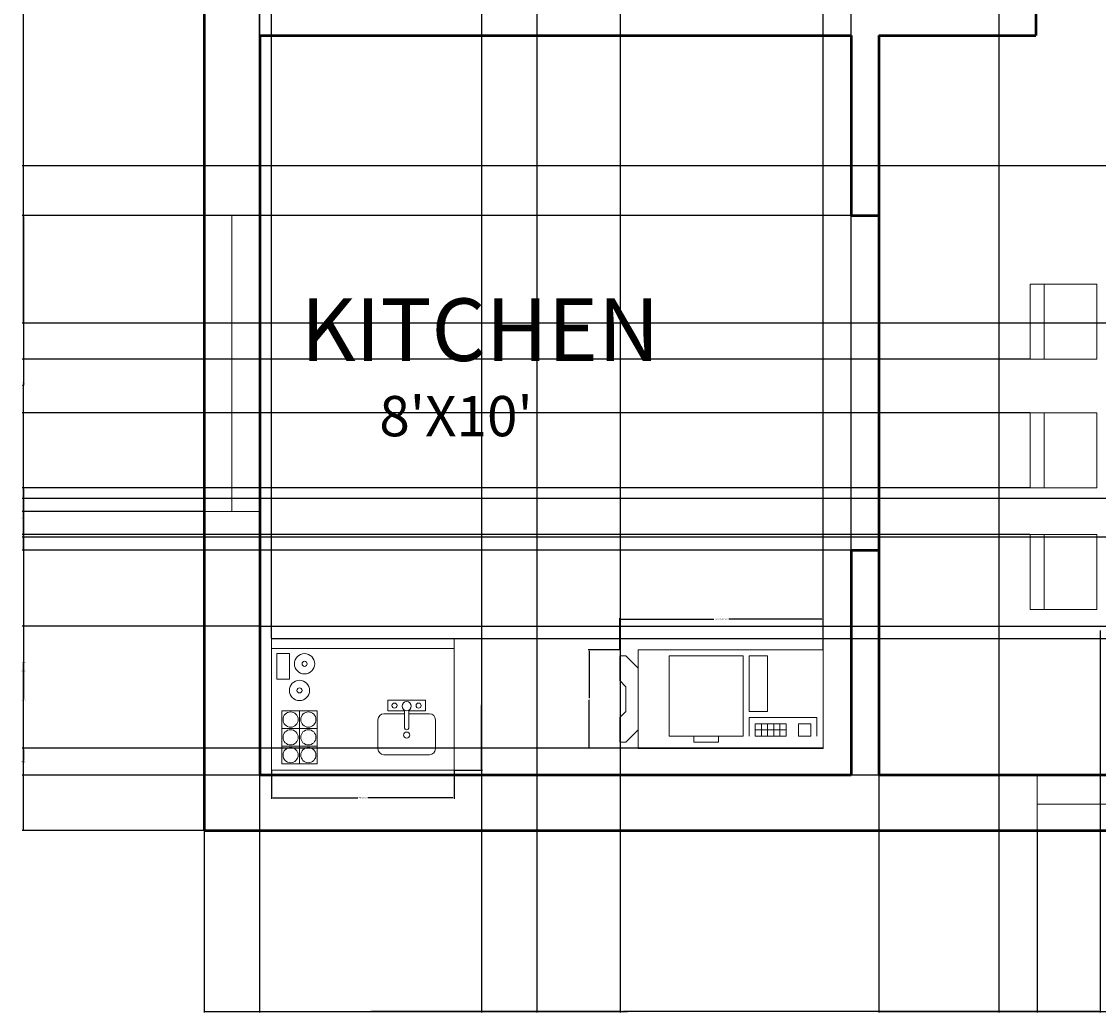
# Model space of a CAD drawing. Units: inches. Extents: x 19425 to 19848, y 45806 to 46417.
# Tile 1 of 5: x 19425 to 19600, y 45806 to 45967. Entities that reach past the tile are written whole.
import ezdxf

# ---------------------------------------------------------------- set-up
doc = ezdxf.new("R2010")
doc.units = ezdxf.units.IN
for name, color, linetype, lineweight in [('A-ANNO-DIMS', 2, 'Continuous', 18), ('A-AREA-IDEN', 3, 'Continuous', 25), ('A-EQPM', 2, 'Continuous', 18), ('A-FLOR-CASE', 2, 'Continuous', 20), ('A-FLOR-FIXT', 2, 'Continuous', 20), ('furniture', 2, 'Continuous', 18), ('wall', 6, 'Continuous', 50), ('window', 9, 'Continuous', 20)]:
    doc.layers.add(name, color=color, linetype=linetype, lineweight=lineweight)
doc.styles.get("Standard").update_dxf_attribs({"font": 'arial.ttf'})
doc.dimstyles.get("Standard").update_dxf_attribs({"dimtxt": 0.18, "dimasz": 0.18, "dimexe": 0.18, "dimexo": 0.0625, "dimgap": 0.09, "dimtad": 0, "dimtih": 1, "dimtoh": 1, "dimdec": 4, "dimzin": 0, "dimdsep": 46, "dimtxsty": 'Standard', "dimcen": 0.09, "dimadec": 0, "dimazin": 0, "dimtfac": 1, "dimtdec": 4, "dimtofl": 0, "dimtmove": 0, "dimatfit": 3, "dimfxl": 1, "dimtolj": 1, "dimtzin": 0, "dimarcsym": 0})

# ---------------------------------------------------------------- blocks, each defined once
blk = doc.blocks.new('Copy Machine')
for p, q in [((0, 0), (0, -16)), ((30, 0), (0, 0)), ((30, -16), (30, 0)), ((-3, -1), (-3, -5)), ((-2, -1), (-3, -1)), ((0, -3), (-2, -1)), ((5, -1), (5, -14)), ((17, -1), (5, -1)), ((17, -14), (17, -1)), ((18, -1), (18, -10)), ((21, -1), (18, -1)), ((21, -10), (21, -1)), ((-3, -5), (-2, -6)), ((-2, -10), (-2, -6)), ((-3, -11), (-2, -10)), ((18, -10), (21, -10)), ((-3, -15), (-3, -11)), ((18, -14), (18, -11)), ((18, -11), (29, -11)), ((24, -12), (19, -12)), ((19, -12), (19, -14)), ((20, -12), (20, -14)), ((21, -14), (21, -12)), ((22, -12), (22, -14)), ((23, -14), (23, -12)), ((24, -14), (24, -12)), ((28, -12), (26, -12)), ((26, -12), (26, -14)), ((28, -14), (28, -12)), ((29, -11), (29, -14)), ((0, -13), (-2, -15)), ((24, -13), (19, -13)), ((-2, -15), (-3, -15)), ((5, -14), (17, -14)), ((9, -14), (9, -15)), ((9, -15), (13, -15)), ((13, -15), (13, -14)), ((19, -14), (24, -14)), ((26, -14), (28, -14)), ((0, -16), (30, -16))]:
    blk.add_line(p, q)
blk = doc.blocks.new('Wet Bar')
for p, q in [((0, 0), (36, 0)), ((0, -26), (0, 0)), ((36, 0), (36, -26)), ((0, -2), (36, -2)), ((3.5, -3), (1, -3)), ((1, -3), (1, -8)), ((3.5, -8), (3.5, -3)), ((1, -8), (3.5, -8)), ((2, -14.25), (9, -14.25)), ((2, -24.75), (2, -14.25)), ((5.5, -14.25), (5.5, -24.75)), ((9, -14.25), (9, -24.75)), ((26.2, -17.55), (26.2, -14.1284)), ((27.1001, -17.55), (27.1001, -14.1284)), ((2, -17.75), (9, -17.75)), ((9, -21.25), (2, -21.25)), ((9, -24.75), (2, -24.75)), ((36, -26), (0, -26))]:
    blk.add_line(p, q)
for points in [[(26.2, -14.25), (22.95, -14.25), (22.95, -12.2), (26.75, -12.2)], [(26.7487, -12.2), (30.3501, -12.2), (30.3501, -14.25), (27.1001, -14.25)], [(22.15, -14.85), (26.2, -14.85)], [(27.1001, -14.85), (31.15, -14.85)], [(20.95, -21.75), (20.95, -16.05)], [(32.3501, -16.05), (32.3501, -21.75)], [(31.15, -22.95), (22.15, -22.95)]]:
    blk.add_lwpolyline(points)
for centre, radius in [((6.5, -5), 2), ((6.5, -5), 0.5), ((5.5, -10.25), 2), ((5.5, -10.25), 0.5), ((26.65, -13.35), 0.9), ((3.75, -16), 1.5), ((7.25, -16), 1.5), ((24.25, -13.25), 0.5), ((29, -13.25), 0.5), ((3.75, -19.5), 1.5), ((7.25, -19.5), 1.5), ((26.65, -19.05), 0.6), ((3.75, -23), 1.5), ((7.25, -23), 1.5)]:
    blk.add_circle(centre, radius)
for centre, radius, start, end in [((22.2251, -16.125), 1.2772, 93.36646, 176.6335), ((31.075, -16.125), 1.2772, 3.366461, 86.63354), ((26.65, -17.55), 0.45, 180, 0), ((22.2251, -21.675), 1.2772, 183.3665, 266.6335), ((31.075, -21.675), 1.2772, 273.3665, 356.6335)]:
    blk.add_arc(centre, radius, start, end)
blk = doc.blocks.new('WIN-48-CENTER-9')
for p, q in [((0, 48), (9, 48)), ((4.5, 0), (4.5, 48)), ((0, 0), (9, 0))]:
    blk.add_line(p, q)
blk = doc.blocks.new('WIN-48-OFFSET-9')
for p, q in [((0, 0), (0, 9)), ((48, 0), (48, 9)), ((48, 4.28), (0, 4.28))]:
    blk.add_line(p, q)
blk = doc.blocks.new('CHAIR-DINING')
blk.add_line((0, 8.53), (12.17, 8.53))
blk.add_lwpolyline([(0, 10.82), (12.17, 10.82), (12.17, 0), (0, 0)], close=True)
blk = doc.blocks.new('*D28')
at = {"layer": 'A-ANNO-DIMS', "color": 0, "lineweight": -2, "transparency": 16777216}
for p, q in [((19522.24, 45865.14), (19522.24, 45870.21)), ((19522.42, 45870.03), (19537.52, 45870.03)), ((19555.06, 45870.03), (19539.96, 45870.03)), ((19555.24, 45865.14), (19555.24, 45870.21))]:
    blk.add_line(p, q, dxfattribs=at)
at = {"layer": 'A-ANNO-DIMS', "color": 0, "transparency": 16777216}
for points in [[(19522.42, 45870.06), (19522.42, 45870), (19522.24, 45870.03)], [(19555.06, 45870.06), (19555.06, 45870), (19555.24, 45870.03)]]:
    blk.add_solid(points, dxfattribs=at)
at = {"layer": 'Defpoints', "color": 0, "transparency": 16777216}
for p in [(19555.24, 45870.03), (19522.24, 45865.08), (19555.24, 45865.08)]:
    blk.add_point(p, dxfattribs=at)
at = {"layer": 'A-ANNO-DIMS', "color": 0, "transparency": 16777216, "insert": (19538.74, 45870.03), "char_height": 0.18, "attachment_point": 5}
blk.add_mtext('\\A1;COPY MACHINE 33', dxfattribs=at)
blk = doc.blocks.new('*D29')
at = {"layer": 'A-ANNO-DIMS', "color": 0, "lineweight": -2, "transparency": 16777216}
for p, q in [((19522.18, 45865.08), (19517.11, 45865.08)), ((19517.29, 45864.9), (19517.29, 45857.26)), ((19517.29, 45849.26), (19517.29, 45856.89)), ((19522.18, 45849.08), (19517.11, 45849.08))]:
    blk.add_line(p, q, dxfattribs=at)
at = {"layer": 'A-ANNO-DIMS', "color": 0, "transparency": 16777216}
for points in [[(19517.26, 45864.9), (19517.32, 45864.9), (19517.29, 45865.08)], [(19517.26, 45849.26), (19517.32, 45849.26), (19517.29, 45849.08)]]:
    blk.add_solid(points, dxfattribs=at)
at = {"layer": 'Defpoints', "color": 0, "transparency": 16777216}
for p in [(19517.29, 45865.08), (19522.24, 45865.08), (19522.24, 45849.08)]:
    blk.add_point(p, dxfattribs=at)
at = {"layer": 'A-ANNO-DIMS', "color": 0, "transparency": 16777216, "insert": (19517.29, 45857.08), "char_height": 0.18, "attachment_point": 5}
blk.add_mtext('\\A1;16', dxfattribs=at)
blk = doc.blocks.new('*D30')
at = {"layer": 'A-ANNO-DIMS', "color": 0, "lineweight": -2, "transparency": 16777216}
for p, q in [((19465.72, 45845.46), (19465.72, 45840.89)), ((19495.34, 45845.46), (19495.34, 45840.89)), ((19465.9, 45841.07), (19479.7, 45841.07)), ((19495.16, 45841.07), (19481.36, 45841.07))]:
    blk.add_line(p, q, dxfattribs=at)
at = {"layer": 'A-ANNO-DIMS', "color": 0, "transparency": 16777216}
for points in [[(19465.9, 45841.1), (19465.9, 45841.04), (19465.72, 45841.07)], [(19495.16, 45841.1), (19495.16, 45841.04), (19495.34, 45841.07)]]:
    blk.add_solid(points, dxfattribs=at)
at = {"layer": 'Defpoints', "color": 0, "transparency": 16777216}
for p in [(19465.72, 45845.52), (19495.34, 45845.52), (19495.34, 45841.07)]:
    blk.add_point(p, dxfattribs=at)
at = {"layer": 'A-ANNO-DIMS', "color": 0, "transparency": 16777216, "insert": (19480.53, 45841.07), "char_height": 0.18, "attachment_point": 5}
blk.add_mtext('\\A1;WET BAR 30', dxfattribs=at)
blk = doc.blocks.new('*D31')
at = {"layer": 'A-ANNO-DIMS', "color": 0, "lineweight": -2, "transparency": 16777216}
for p, q in [((19495.4, 45866.91), (19499.96, 45866.91)), ((19499.78, 45866.73), (19499.78, 45856.39)), ((19499.78, 45845.7), (19499.78, 45856.03)), ((19495.4, 45845.52), (19499.96, 45845.52))]:
    blk.add_line(p, q, dxfattribs=at)
at = {"layer": 'A-ANNO-DIMS', "color": 0, "transparency": 16777216}
for points in [[(19499.75, 45866.73), (19499.81, 45866.73), (19499.78, 45866.91)], [(19499.75, 45845.7), (19499.81, 45845.7), (19499.78, 45845.52)]]:
    blk.add_solid(points, dxfattribs=at)
at = {"layer": 'Defpoints', "color": 0, "transparency": 16777216}
for p in [(19495.34, 45866.91), (19499.78, 45866.91), (19495.34, 45845.52)]:
    blk.add_point(p, dxfattribs=at)
at = {"layer": 'A-ANNO-DIMS', "color": 0, "transparency": 16777216, "insert": (19499.78, 45856.21), "char_height": 0.18, "attachment_point": 5}
blk.add_mtext('\\A1;21', dxfattribs=at)
blk = doc.blocks.new('*D34')
at = {"layer": 'A-ANNO-DIMS', "color": 0, "lineweight": -2, "transparency": 16777216}
for p, q in [((19522.3, 46304.14), (19522.3, 45806.22)), ((19463.78, 46303.69), (19463.78, 45806.22)), ((19463.96, 45806.4), (19492.65, 45806.4)), ((19522.12, 45806.4), (19493.43, 45806.4))]:
    blk.add_line(p, q, dxfattribs=at)
at = {"layer": 'A-ANNO-DIMS', "color": 0, "transparency": 16777216}
for points in [[(19463.96, 45806.43), (19463.96, 45806.37), (19463.78, 45806.4)], [(19522.12, 45806.43), (19522.12, 45806.37), (19522.3, 45806.4)]]:
    blk.add_solid(points, dxfattribs=at)
at = {"layer": 'Defpoints', "color": 0, "transparency": 16777216}
for p in [(19522.3, 46304.2), (19463.78, 46303.75), (19522.3, 45806.4)]:
    blk.add_point(p, dxfattribs=at)
at = {"layer": 'A-ANNO-DIMS', "color": 0, "transparency": 16777216, "insert": (19493.04, 45806.4), "char_height": 0.18, "attachment_point": 5}
blk.add_mtext('\\A1;58.52', dxfattribs=at)
blk = doc.blocks.new('*D37')
at = {"layer": 'A-ANNO-DIMS', "color": 0, "lineweight": -2, "transparency": 16777216}
for p, q in [((19454.72, 45887.51), (19425.25, 45887.51)), ((19425.43, 45887.33), (19425.43, 45861.82)), ((19425.43, 45835.93), (19425.43, 45861.45)), ((19454.72, 45835.75), (19425.25, 45835.75))]:
    blk.add_line(p, q, dxfattribs=at)
at = {"layer": 'A-ANNO-DIMS', "color": 0, "transparency": 16777216}
for points in [[(19425.4, 45887.33), (19425.46, 45887.33), (19425.43, 45887.51)], [(19425.4, 45835.93), (19425.46, 45835.93), (19425.43, 45835.75)]]:
    blk.add_solid(points, dxfattribs=at)
at = {"layer": 'Defpoints', "color": 0, "transparency": 16777216}
for p in [(19425.43, 45887.51), (19454.78, 45887.51), (19454.78, 45835.75)]:
    blk.add_point(p, dxfattribs=at)
at = {"layer": 'A-ANNO-DIMS', "color": 0, "transparency": 16777216, "insert": (19425.43, 45861.63), "char_height": 0.18, "attachment_point": 5}
blk.add_mtext('\\A1;51.76', dxfattribs=at)
blk = doc.blocks.new('*D38')
at = {"layer": 'A-ANNO-DIMS', "color": 0, "lineweight": -2, "transparency": 16777216}
for p, q in [((19808.72, 45889.62), (19425.25, 45889.62)), ((19425.43, 45889.44), (19425.43, 45886.67)), ((19425.43, 45883.53), (19425.43, 45886.3)), ((19802.72, 45883.35), (19425.25, 45883.35))]:
    blk.add_line(p, q, dxfattribs=at)
at = {"layer": 'A-ANNO-DIMS', "color": 0, "transparency": 16777216}
for points in [[(19425.4, 45889.44), (19425.46, 45889.44), (19425.43, 45889.62)], [(19425.4, 45883.53), (19425.46, 45883.53), (19425.43, 45883.35)]]:
    blk.add_solid(points, dxfattribs=at)
at = {"layer": 'Defpoints', "color": 0, "transparency": 16777216}
for p in [(19425.43, 45889.62), (19808.78, 45889.62), (19802.78, 45883.35)]:
    blk.add_point(p, dxfattribs=at)
at = {"layer": 'A-ANNO-DIMS', "color": 0, "transparency": 16777216, "insert": (19425.43, 45886.49), "char_height": 0.18, "attachment_point": 5}
blk.add_mtext('\\A1;6.261', dxfattribs=at)
blk = doc.blocks.new('*D39')
at = {"layer": 'A-ANNO-DIMS', "color": 0, "lineweight": -2, "transparency": 16777216}
for p, q in [((19454.78, 45835.69), (19454.78, 45806.22)), ((19590, 45835.69), (19590, 45806.22)), ((19454.96, 45806.4), (19521.93, 45806.4)), ((19589.82, 45806.4), (19522.84, 45806.4))]:
    blk.add_line(p, q, dxfattribs=at)
at = {"layer": 'A-ANNO-DIMS', "color": 0, "transparency": 16777216}
for points in [[(19454.96, 45806.43), (19454.96, 45806.37), (19454.78, 45806.4)], [(19589.82, 45806.43), (19589.82, 45806.37), (19590, 45806.4)]]:
    blk.add_solid(points, dxfattribs=at)
at = {"layer": 'Defpoints', "color": 0, "transparency": 16777216}
for p in [(19454.78, 45835.75), (19590, 45835.75), (19590, 45806.4)]:
    blk.add_point(p, dxfattribs=at)
at = {"layer": 'A-ANNO-DIMS', "color": 0, "transparency": 16777216, "insert": (19522.39, 45806.4), "char_height": 0.18, "attachment_point": 5}
blk.add_mtext('\\A1;135.22', dxfattribs=at)
blk = doc.blocks.new('*D43')
at = {"layer": 'A-ANNO-DIMS', "color": 0, "lineweight": -2, "transparency": 16777216}
for p, q in [((19564.28, 45844.69), (19564.28, 45806.22)), ((19666.28, 45844.69), (19666.28, 45806.22)), ((19564.46, 45806.4), (19615, 45806.4)), ((19666.1, 45806.4), (19615.56, 45806.4))]:
    blk.add_line(p, q, dxfattribs=at)
at = {"layer": 'A-ANNO-DIMS', "color": 0, "transparency": 16777216}
for points in [[(19564.46, 45806.43), (19564.46, 45806.37), (19564.28, 45806.4)], [(19666.1, 45806.43), (19666.1, 45806.37), (19666.28, 45806.4)]]:
    blk.add_solid(points, dxfattribs=at)
at = {"layer": 'Defpoints', "color": 0, "transparency": 16777216}
for p in [(19564.28, 45844.75), (19666.28, 45844.75), (19666.28, 45806.4)]:
    blk.add_point(p, dxfattribs=at)
at = {"layer": 'A-ANNO-DIMS', "color": 0, "transparency": 16777216, "insert": (19615.28, 45806.4), "char_height": 0.18, "attachment_point": 5}
blk.add_mtext('\\A1;102', dxfattribs=at)
blk = doc.blocks.new('*D48')
at = {"layer": 'A-ANNO-DIMS', "color": 0, "lineweight": -2, "transparency": 16777216}
for p, q in [((19564.22, 45935.54), (19425.25, 45935.54)), ((19425.43, 45935.36), (19425.43, 45908.56)), ((19425.43, 45881.4), (19425.43, 45908.19)), ((19564.22, 45881.22), (19425.25, 45881.22))]:
    blk.add_line(p, q, dxfattribs=at)
at = {"layer": 'A-ANNO-DIMS', "color": 0, "transparency": 16777216}
for points in [[(19425.4, 45935.36), (19425.46, 45935.36), (19425.43, 45935.54)], [(19425.4, 45881.4), (19425.46, 45881.4), (19425.43, 45881.22)]]:
    blk.add_solid(points, dxfattribs=at)
at = {"layer": 'Defpoints', "color": 0, "transparency": 16777216}
for p in [(19425.43, 45935.54), (19564.28, 45935.54), (19564.28, 45881.22)]:
    blk.add_point(p, dxfattribs=at)
at = {"layer": 'A-ANNO-DIMS', "color": 0, "transparency": 16777216, "insert": (19425.43, 45908.38), "char_height": 0.18, "attachment_point": 5}
blk.add_mtext('\\A1;54.32', dxfattribs=at)
blk = doc.blocks.new('*D52')
at = {"layer": 'A-ANNO-DIMS', "color": 0, "lineweight": -2, "transparency": 16777216}
for p, q in [((19732.81, 46000.63), (19425.25, 46000.63)), ((19425.43, 46000.45), (19425.43, 45972.3)), ((19425.43, 45943.79), (19425.43, 45971.94)), ((19732.81, 45943.61), (19425.25, 45943.61))]:
    blk.add_line(p, q, dxfattribs=at)
at = {"layer": 'A-ANNO-DIMS', "color": 0, "transparency": 16777216}
for points in [[(19425.4, 46000.45), (19425.46, 46000.45), (19425.43, 46000.63)], [(19425.4, 45943.79), (19425.46, 45943.79), (19425.43, 45943.61)]]:
    blk.add_solid(points, dxfattribs=at)
at = {"layer": 'Defpoints', "color": 0, "transparency": 16777216}
for p in [(19425.43, 46000.63), (19732.87, 46000.63), (19732.87, 45943.61)]:
    blk.add_point(p, dxfattribs=at)
at = {"layer": 'A-ANNO-DIMS', "color": 0, "transparency": 16777216, "insert": (19425.43, 45972.12), "char_height": 0.18, "attachment_point": 5}
blk.add_mtext('\\A1;57.02', dxfattribs=at)
blk = doc.blocks.new('*D54')
at = {"layer": 'A-ANNO-DIMS', "color": 0, "lineweight": -2, "transparency": 16777216}
for p, q in [((19808.72, 46048.75), (19425.25, 46048.75)), ((19425.43, 46048.57), (19425.43, 45983.58)), ((19425.43, 45918.22), (19425.43, 45983.22)), ((19808.72, 45918.04), (19425.25, 45918.04))]:
    blk.add_line(p, q, dxfattribs=at)
at = {"layer": 'A-ANNO-DIMS', "color": 0, "transparency": 16777216}
for points in [[(19425.4, 46048.57), (19425.46, 46048.57), (19425.43, 46048.75)], [(19425.4, 45918.22), (19425.46, 45918.22), (19425.43, 45918.04)]]:
    blk.add_solid(points, dxfattribs=at)
at = {"layer": 'Defpoints', "color": 0, "transparency": 16777216}
for p in [(19425.43, 46048.75), (19808.78, 46048.75), (19808.78, 45918.04)]:
    blk.add_point(p, dxfattribs=at)
at = {"layer": 'A-ANNO-DIMS', "color": 0, "transparency": 16777216, "insert": (19425.43, 45983.4), "char_height": 0.18, "attachment_point": 5}
blk.add_mtext('\\A1;130.7', dxfattribs=at)
blk = doc.blocks.new('*D56')
at = {"layer": 'A-ANNO-DIMS', "color": 0, "lineweight": -2, "transparency": 16777216}
for p, q in [((19564.28, 45881.15), (19564.28, 45806.22)), ((19600.2, 45868.22), (19600.2, 45806.22)), ((19564.46, 45806.4), (19581.85, 45806.4)), ((19600.02, 45806.4), (19582.63, 45806.4))]:
    blk.add_line(p, q, dxfattribs=at)
at = {"layer": 'A-ANNO-DIMS', "color": 0, "transparency": 16777216}
for points in [[(19564.46, 45806.43), (19564.46, 45806.37), (19564.28, 45806.4)], [(19600.02, 45806.43), (19600.02, 45806.37), (19600.2, 45806.4)]]:
    blk.add_solid(points, dxfattribs=at)
at = {"layer": 'Defpoints', "color": 0, "transparency": 16777216}
for p in [(19564.28, 45881.22), (19600.2, 45868.28), (19600.2, 45806.4)]:
    blk.add_point(p, dxfattribs=at)
at = {"layer": 'A-ANNO-DIMS', "color": 0, "transparency": 16777216, "insert": (19582.24, 45806.4), "char_height": 0.18, "attachment_point": 5}
blk.add_mtext('\\A1;35.92', dxfattribs=at)
blk = doc.blocks.new('*D58')
at = {"layer": 'A-ANNO-DIMS', "color": 0, "lineweight": -2, "transparency": 16777216}
for p, q in [((19463.72, 45868.92), (19425.25, 45868.92)), ((19425.43, 45868.74), (19425.43, 45857.02)), ((19425.43, 45844.93), (19425.43, 45856.65)), ((19463.72, 45844.75), (19425.25, 45844.75))]:
    blk.add_line(p, q, dxfattribs=at)
at = {"layer": 'A-ANNO-DIMS', "color": 0, "transparency": 16777216}
for points in [[(19425.4, 45868.74), (19425.46, 45868.74), (19425.43, 45868.92)], [(19425.4, 45844.93), (19425.46, 45844.93), (19425.43, 45844.75)]]:
    blk.add_solid(points, dxfattribs=at)
at = {"layer": 'Defpoints', "color": 0, "transparency": 16777216}
for p in [(19425.43, 45868.92), (19463.78, 45868.92), (19463.78, 45844.75)]:
    blk.add_point(p, dxfattribs=at)
at = {"layer": 'A-ANNO-DIMS', "color": 0, "transparency": 16777216, "insert": (19425.43, 45856.84), "char_height": 0.18, "attachment_point": 5}
blk.add_mtext('\\A1;24.16', dxfattribs=at)
blk = doc.blocks.new('*D59')
at = {"layer": 'A-ANNO-DIMS', "color": 0, "lineweight": -2, "transparency": 16777216}
for p, q in [((19463.78, 45868.98), (19463.78, 46342.28)), ((19463.96, 46342.1), (19464.36, 46342.1)), ((19465.54, 46342.1), (19465.14, 46342.1)), ((19465.72, 45866.97), (19465.72, 46342.28))]:
    blk.add_line(p, q, dxfattribs=at)
at = {"layer": 'A-ANNO-DIMS', "color": 0, "transparency": 16777216}
for points in [[(19463.96, 46342.13), (19463.96, 46342.07), (19463.78, 46342.1)], [(19465.54, 46342.13), (19465.54, 46342.07), (19465.72, 46342.1)]]:
    blk.add_solid(points, dxfattribs=at)
at = {"layer": 'Defpoints', "color": 0, "transparency": 16777216}
for p in [(19465.72, 46342.1), (19463.78, 45868.92), (19465.72, 45866.91)]:
    blk.add_point(p, dxfattribs=at)
at = {"layer": 'A-ANNO-DIMS', "color": 0, "transparency": 16777216, "insert": (19464.75, 46342.1), "char_height": 0.18, "attachment_point": 5}
blk.add_mtext('\\A1;1.938', dxfattribs=at)
blk = doc.blocks.new('*D60')
at = {"layer": 'A-ANNO-DIMS', "color": 0, "lineweight": -2, "transparency": 16777216}
for p, q in [((19555.24, 45865.14), (19555.24, 46342.28)), ((19555.42, 46342.1), (19557.18, 46342.1)), ((19559.6, 46342.1), (19557.84, 46342.1)), ((19559.78, 45868.98), (19559.78, 46342.28))]:
    blk.add_line(p, q, dxfattribs=at)
at = {"layer": 'A-ANNO-DIMS', "color": 0, "transparency": 16777216}
for points in [[(19555.42, 46342.13), (19555.42, 46342.07), (19555.24, 46342.1)], [(19559.6, 46342.13), (19559.6, 46342.07), (19559.78, 46342.1)]]:
    blk.add_solid(points, dxfattribs=at)
at = {"layer": 'Defpoints', "color": 0, "transparency": 16777216}
for p in [(19559.78, 46342.1), (19559.78, 45868.92), (19555.24, 45865.08)]:
    blk.add_point(p, dxfattribs=at)
at = {"layer": 'A-ANNO-DIMS', "color": 0, "transparency": 16777216, "insert": (19557.51, 46342.1), "char_height": 0.18, "attachment_point": 5}
blk.add_mtext('\\A1;4.54', dxfattribs=at)
blk = doc.blocks.new('*D63')
at = {"layer": 'A-ANNO-DIMS', "color": 0, "lineweight": -2, "transparency": 16777216}
for p, q in [((19463.78, 46125.19), (19463.78, 45806.22)), ((19583.78, 46125.19), (19583.78, 45806.22)), ((19463.96, 45806.4), (19523.5, 45806.4)), ((19583.6, 45806.4), (19524.06, 45806.4))]:
    blk.add_line(p, q, dxfattribs=at)
at = {"layer": 'A-ANNO-DIMS', "color": 0, "transparency": 16777216}
for points in [[(19463.96, 45806.43), (19463.96, 45806.37), (19463.78, 45806.4)], [(19583.6, 45806.43), (19583.6, 45806.37), (19583.78, 45806.4)]]:
    blk.add_solid(points, dxfattribs=at)
at = {"layer": 'Defpoints', "color": 0, "transparency": 16777216}
for p in [(19463.78, 46125.25), (19583.78, 46125.25), (19583.78, 45806.4)]:
    blk.add_point(p, dxfattribs=at)
at = {"layer": 'A-ANNO-DIMS', "color": 0, "transparency": 16777216, "insert": (19523.78, 45806.4), "char_height": 0.18, "attachment_point": 5}
blk.add_mtext('\\A1;120', dxfattribs=at)
blk = doc.blocks.new('*D64')
at = {"layer": 'A-ANNO-DIMS', "color": 0, "lineweight": -2, "transparency": 16777216}
for p, q in [((19463.78, 46048.69), (19463.78, 45806.22)), ((19499.78, 46048.69), (19499.78, 45806.22)), ((19463.96, 45806.4), (19481.56, 45806.4)), ((19499.6, 45806.4), (19482, 45806.4))]:
    blk.add_line(p, q, dxfattribs=at)
at = {"layer": 'A-ANNO-DIMS', "color": 0, "transparency": 16777216}
for points in [[(19463.96, 45806.43), (19463.96, 45806.37), (19463.78, 45806.4)], [(19499.6, 45806.43), (19499.6, 45806.37), (19499.78, 45806.4)]]:
    blk.add_solid(points, dxfattribs=at)
at = {"layer": 'Defpoints', "color": 0, "transparency": 16777216}
for p in [(19463.78, 46048.75), (19499.78, 46048.75), (19499.78, 45806.4)]:
    blk.add_point(p, dxfattribs=at)
at = {"layer": 'A-ANNO-DIMS', "color": 0, "transparency": 16777216, "insert": (19481.78, 45806.4), "char_height": 0.18, "attachment_point": 5}
blk.add_mtext('\\A1;36', dxfattribs=at)
blk = doc.blocks.new('*D65')
at = {"layer": 'A-ANNO-DIMS', "color": 0, "lineweight": -2, "transparency": 16777216}
for p, q in [((19499.78, 46048.69), (19499.78, 45806.22)), ((19508.78, 46048.69), (19508.78, 45806.22)), ((19499.96, 45806.4), (19504.13, 45806.4)), ((19508.6, 45806.4), (19504.43, 45806.4))]:
    blk.add_line(p, q, dxfattribs=at)
at = {"layer": 'A-ANNO-DIMS', "color": 0, "transparency": 16777216}
for points in [[(19499.96, 45806.43), (19499.96, 45806.37), (19499.78, 45806.4)], [(19508.6, 45806.43), (19508.6, 45806.37), (19508.78, 45806.4)]]:
    blk.add_solid(points, dxfattribs=at)
at = {"layer": 'Defpoints', "color": 0, "transparency": 16777216}
for p in [(19499.78, 46048.75), (19508.78, 46048.75), (19508.78, 45806.4)]:
    blk.add_point(p, dxfattribs=at)
at = {"layer": 'A-ANNO-DIMS', "color": 0, "transparency": 16777216, "insert": (19504.28, 45806.4), "char_height": 0.18, "attachment_point": 5}
blk.add_mtext('\\A1;9', dxfattribs=at)
blk = doc.blocks.new('*D71')
at = {"layer": 'A-ANNO-DIMS', "color": 0, "lineweight": -2, "transparency": 16777216}
for p, q in [((19564.22, 45881.22), (19425.25, 45881.22)), ((19425.43, 45881.04), (19425.43, 45863.17)), ((19425.43, 45844.93), (19425.43, 45862.8)), ((19564.22, 45844.75), (19425.25, 45844.75))]:
    blk.add_line(p, q, dxfattribs=at)
at = {"layer": 'A-ANNO-DIMS', "color": 0, "transparency": 16777216}
for points in [[(19425.4, 45881.04), (19425.46, 45881.04), (19425.43, 45881.22)], [(19425.4, 45844.93), (19425.46, 45844.93), (19425.43, 45844.75)]]:
    blk.add_solid(points, dxfattribs=at)
at = {"layer": 'Defpoints', "color": 0, "transparency": 16777216}
for p in [(19425.43, 45881.22), (19564.28, 45881.22), (19564.28, 45844.75)]:
    blk.add_point(p, dxfattribs=at)
at = {"layer": 'A-ANNO-DIMS', "color": 0, "transparency": 16777216, "insert": (19425.43, 45862.99), "char_height": 0.18, "attachment_point": 5}
blk.add_mtext('\\A1;36.46', dxfattribs=at)
blk = doc.blocks.new('*D72')
at = {"layer": 'A-ANNO-DIMS', "color": 0, "lineweight": -2, "transparency": 16777216}
for p, q in [((19588.8, 45912.22), (19425.25, 45912.22)), ((19425.43, 45912.04), (19425.43, 45908.06)), ((19425.43, 45903.71), (19425.43, 45907.7)), ((19588.8, 45903.53), (19425.25, 45903.53))]:
    blk.add_line(p, q, dxfattribs=at)
at = {"layer": 'A-ANNO-DIMS', "color": 0, "transparency": 16777216}
for points in [[(19425.4, 45912.04), (19425.46, 45912.04), (19425.43, 45912.22)], [(19425.4, 45903.71), (19425.46, 45903.71), (19425.43, 45903.53)]]:
    blk.add_solid(points, dxfattribs=at)
at = {"layer": 'Defpoints', "color": 0, "transparency": 16777216}
for p in [(19425.43, 45912.22), (19588.86, 45912.22), (19588.86, 45903.53)]:
    blk.add_point(p, dxfattribs=at)
at = {"layer": 'A-ANNO-DIMS', "color": 0, "transparency": 16777216, "insert": (19425.43, 45907.88), "char_height": 0.18, "attachment_point": 5}
blk.add_mtext('\\A1;8.69', dxfattribs=at)
blk = doc.blocks.new('*D73')
at = {"layer": 'A-ANNO-DIMS', "color": 0, "lineweight": -2, "transparency": 16777216}
for p, q in [((19588.8, 45891.36), (19425.25, 45891.36)), ((19425.43, 45891.18), (19425.43, 45887.74)), ((19425.43, 45883.93), (19425.43, 45887.38)), ((19588.8, 45883.75), (19425.25, 45883.75))]:
    blk.add_line(p, q, dxfattribs=at)
at = {"layer": 'A-ANNO-DIMS', "color": 0, "transparency": 16777216}
for points in [[(19425.4, 45891.18), (19425.46, 45891.18), (19425.43, 45891.36)], [(19425.4, 45883.93), (19425.46, 45883.93), (19425.43, 45883.75)]]:
    blk.add_solid(points, dxfattribs=at)
at = {"layer": 'Defpoints', "color": 0, "transparency": 16777216}
for p in [(19425.43, 45891.36), (19588.86, 45891.36), (19588.86, 45883.75)]:
    blk.add_point(p, dxfattribs=at)
at = {"layer": 'A-ANNO-DIMS', "color": 0, "transparency": 16777216, "insert": (19425.43, 45887.56), "char_height": 0.18, "attachment_point": 5}
blk.add_mtext('\\A1;7.606', dxfattribs=at)
blk = doc.blocks.new('*D76')
at = {"layer": 'A-ANNO-DIMS', "color": 0, "lineweight": -2, "transparency": 16777216}
for p, q in [((19463.84, 45868.92), (19847.31, 45868.92)), ((19847.13, 45868.74), (19847.13, 45868.09)), ((19847.13, 45867.09), (19847.13, 45867.73)), ((19465.78, 45866.91), (19847.31, 45866.91))]:
    blk.add_line(p, q, dxfattribs=at)
at = {"layer": 'A-ANNO-DIMS', "color": 0, "transparency": 16777216}
for points in [[(19847.1, 45868.74), (19847.16, 45868.74), (19847.13, 45868.92)], [(19847.1, 45867.09), (19847.16, 45867.09), (19847.13, 45866.91)]]:
    blk.add_solid(points, dxfattribs=at)
at = {"layer": 'Defpoints', "color": 0, "transparency": 16777216}
for p in [(19463.78, 45868.92), (19465.72, 45866.91), (19847.13, 45866.91)]:
    blk.add_point(p, dxfattribs=at)
at = {"layer": 'A-ANNO-DIMS', "color": 0, "transparency": 16777216, "insert": (19847.13, 45867.91), "char_height": 0.18, "attachment_point": 5}
blk.add_mtext('\\A1;2.01', dxfattribs=at)
blk = doc.blocks.new('*D77')
at = {"layer": 'A-ANNO-DIMS', "color": 0, "lineweight": -2, "transparency": 16777216}
for p, q in [((19555.18, 45849.08), (19425.25, 45849.08)), ((19425.43, 45848.9), (19425.43, 45847.1)), ((19425.43, 45844.93), (19425.43, 45846.73)), ((19559.72, 45844.75), (19425.25, 45844.75))]:
    blk.add_line(p, q, dxfattribs=at)
at = {"layer": 'A-ANNO-DIMS', "color": 0, "transparency": 16777216}
for points in [[(19425.4, 45848.9), (19425.46, 45848.9), (19425.43, 45849.08)], [(19425.4, 45844.93), (19425.46, 45844.93), (19425.43, 45844.75)]]:
    blk.add_solid(points, dxfattribs=at)
at = {"layer": 'Defpoints', "color": 0, "transparency": 16777216}
for p in [(19555.24, 45849.08), (19425.43, 45844.75), (19559.78, 45844.75)]:
    blk.add_point(p, dxfattribs=at)
at = {"layer": 'A-ANNO-DIMS', "color": 0, "transparency": 16777216, "insert": (19425.43, 45846.92), "char_height": 0.18, "attachment_point": 5}
blk.add_mtext('\\A1;4.321', dxfattribs=at)

msp = doc.modelspace()

# ---------------------------------------------------------------- linework, layer by layer
at = {"layer": 'A-FLOR-CASE'}
msp.add_line((19559.7812, 45868.9163), (19463.7812, 45868.9163), dxfattribs=at)
at = {"layer": 'wall'}
for p, q in [((19454.7812, 46312.7547), (19454.7812, 45835.7547)), ((19589.7812, 45969.2547), (19589.7812, 45964.7547)), ((19463.7812, 45964.7547), (19559.7812, 45964.7547)), ((19463.7812, 45964.7547), (19463.7812, 45844.7547)), ((19559.7812, 45964.7547), (19559.7812, 45935.5363)), ((19564.2812, 45964.7547), (19564.2812, 45844.7547)), ((19564.2812, 45964.7547), (19589.7812, 45964.7547)), ((19559.7812, 45935.5363), (19564.2812, 45935.5363)), ((19559.7812, 45881.2164), (19564.2812, 45881.2164)), ((19559.7812, 45881.2164), (19559.7812, 45844.7547)), ((19463.7812, 45844.7547), (19559.7812, 45844.7547)), ((19564.2812, 45844.7547), (19666.2812, 45844.7547)), ((19454.7812, 45835.7547), (19760.7812, 45835.7547))]:
    msp.add_line(p, q, dxfattribs=at)

# ---------------------------------------------------------------- block references
at = {"layer": 'A-EQPM'}
msp.add_blockref('Copy Machine', (19525.2409, 45865.0758), dxfattribs=at)
at = {"layer": 'A-FLOR-FIXT', "xscale": 0.8227343894153213, "yscale": 0.8227343894153213, "zscale": 0.8227343894153213}
msp.add_blockref('Wet Bar', (19465.7192, 45866.9088), dxfattribs=at)
at = {"layer": 'furniture', "extrusion": (0, 0, -1), "zscale": -1}
for p, rotation in [((-19599.6828, 45924.3969), 269.9999999999708), ((-19599.6828, 45903.5339), 269.9999999999408), ((-19599.6828, 45883.7546), 269.9999999999408)]:
    msp.add_blockref('CHAIR-DINING', p, dxfattribs=dict(at, rotation=rotation))
at = {"layer": 'window'}
for name, p in [('WIN-48-CENTER-9', (19454.7812, 45887.5125)), ('WIN-48-OFFSET-9', (19589.9971, 45835.7547))]:
    msp.add_blockref(name, p, dxfattribs=at)

# ---------------------------------------------------------------- texts
at = {"layer": 'A-AREA-IDEN'}
for s, height, p in [('KITCHEN', 10.12861, (19470.4207, 45911.9395)), ("8'X10'", 6.53608, (19483.201, 45899.7134))]:
    msp.add_text(s, height=height, dxfattribs=at).set_placement(p)

# ---------------------------------------------------------------- dimensions: what is measured, and where the dimension line sits
at = {"layer": 'A-ANNO-DIMS'}
for base, p1, p2, override, picture, middle in [((19465.7192, 46342.1047), (19463.7812, 45868.9163), (19465.7192, 45866.9088), {"dimdec": 3, "dimlfac": 1, "dimrnd": 0, "dimzin": 0, "dimdsep": 46, "dimlunit": 2}, '*D59', (19464.7502, 46342.1047)), ((19559.7812, 46342.1047), (19555.2409, 45865.0758), (19559.7812, 45868.9163), {"dimdec": 2, "dimlfac": 1, "dimrnd": 0, "dimzin": 0, "dimdsep": 46, "dimlunit": 2}, '*D60', (19557.511, 46342.1047)), ((19522.3015, 45806.4047), (19463.7812, 46303.7547), (19522.3015, 46304.1988), {"dimdec": 2, "dimlfac": 1, "dimrnd": 0, "dimzin": 0, "dimdsep": 46, "dimlunit": 2}, '*D34', (19493.0413, 45806.4047)), ((19583.7812, 45806.4047), (19463.7812, 46125.2547), (19583.7812, 46125.2547), {"dimdec": 0, "dimlfac": 1, "dimrnd": 0, "dimzin": 0, "dimdsep": 46, "dimlunit": 2}, '*D63', (19523.7812, 45806.4047)), ((19499.7812, 45806.4047), (19463.7812, 46048.7547), (19499.7812, 46048.7547), {"dimdec": 0, "dimlfac": 1, "dimrnd": 0, "dimzin": 0, "dimdsep": 46, "dimlunit": 2}, '*D64', (19481.7812, 45806.4047)), ((19508.7812, 45806.4047), (19499.7812, 46048.7547), (19508.7812, 46048.7547), {"dimdec": 0, "dimlfac": 1, "dimrnd": 0, "dimzin": 0, "dimdsep": 46, "dimlunit": 2}, '*D65', (19504.2812, 45806.4047)), ((19600.2018, 45806.4047), (19564.2812, 45881.2164), (19600.2018, 45868.2782), {"dimdec": 2, "dimlfac": 1, "dimrnd": 0, "dimzin": 0, "dimdsep": 46, "dimlunit": 2}, '*D56', (19582.2415, 45806.4047)), ((19666.2812, 45806.4047), (19564.2812, 45844.7547), (19666.2812, 45844.7547), {"dimdec": 0, "dimlfac": 1, "dimrnd": 0, "dimzin": 0, "dimdsep": 46, "dimlunit": 2}, '*D43', (19615.2812, 45806.4047)), ((19589.9971, 45806.4047), (19454.7812, 45835.7547), (19589.9971, 45835.7547), {"dimdec": 2, "dimlfac": 1, "dimrnd": 0, "dimzin": 0, "dimdsep": 46, "dimlunit": 2}, '*D39', (19522.3891, 45806.4047))]:
    dim = msp.add_linear_dim(base=base, p1=p1, p2=p2, dimstyle='Standard', override=override, dxfattribs=at)
    dim.commit()
    dim.dimension.update_dxf_attribs({"geometry": picture, "text_midpoint": middle})
for base, p1, p2, override, picture, middle in [((19425.4312, 46048.7547), (19808.7812, 45918.0438), (19808.7812, 46048.7547), {"dimdec": 1, "dimlfac": 1, "dimrnd": 0, "dimzin": 0, "dimdsep": 46, "dimlunit": 2}, '*D54', (19425.4312, 45983.3992)), ((19425.4312, 46000.631), (19732.8741, 45943.6092), (19732.8741, 46000.631), {"dimdec": 2, "dimlfac": 1, "dimrnd": 0, "dimzin": 0, "dimdsep": 46, "dimlunit": 2}, '*D52', (19425.4312, 45972.1201)), ((19425.4312, 45935.5363), (19564.2812, 45881.2164), (19564.2812, 45935.5363), {"dimdec": 2, "dimlfac": 1, "dimrnd": 0, "dimzin": 0, "dimdsep": 46, "dimlunit": 2}, '*D48', (19425.4312, 45908.3763)), ((19425.4312, 45912.2237), (19588.864, 45903.5339), (19588.864, 45912.2237), {"dimdec": 2, "dimlfac": 1, "dimrnd": 0, "dimzin": 0, "dimdsep": 46, "dimlunit": 2}, '*D72', (19425.4312, 45907.8788)), ((19425.4312, 45891.3607), (19588.864, 45883.7546), (19588.864, 45891.3607), {"dimdec": 3, "dimlfac": 1, "dimrnd": 0, "dimzin": 0, "dimdsep": 46, "dimlunit": 2}, '*D73', (19425.4312, 45887.5577)), ((19425.4312, 45889.6159), (19802.7812, 45883.3547), (19808.7812, 45889.6159), {"dimdec": 3, "dimlfac": 1, "dimrnd": 0, "dimzin": 0, "dimdsep": 46, "dimlunit": 2}, '*D38', (19425.4312, 45886.4853)), ((19425.4312, 45887.5125), (19454.7812, 45835.7547), (19454.7812, 45887.5125), {"dimdec": 2, "dimlfac": 1, "dimrnd": 0, "dimzin": 0, "dimdsep": 46, "dimlunit": 2}, '*D37', (19425.4312, 45861.6336)), ((19425.4312, 45881.2164), (19564.2812, 45844.7547), (19564.2812, 45881.2164), {"dimdec": 2, "dimlfac": 1, "dimrnd": 0, "dimzin": 0, "dimdsep": 46, "dimlunit": 2}, '*D71', (19425.4312, 45862.9855)), ((19425.4312, 45868.9163), (19463.7812, 45844.7547), (19463.7812, 45868.9163), {"dimdec": 2, "dimlfac": 1, "dimrnd": 0, "dimzin": 0, "dimdsep": 46, "dimlunit": 2}, '*D58', (19425.4312, 45856.8355)), ((19847.1312, 45866.9088), (19463.7812, 45868.9163), (19465.7192, 45866.9088), {"dimdec": 2, "dimlfac": 1, "dimrnd": 0, "dimzin": 0, "dimdsep": 46, "dimlunit": 2}, '*D76', (19847.1312, 45867.9126)), ((19499.7804, 45866.9088), (19495.3377, 45845.5177), (19495.3377, 45866.9088), {"dimdec": 0, "dimlfac": 1, "dimrnd": 0, "dimzin": 0, "dimdsep": 46, "dimlunit": 2}, '*D31', (19499.7804, 45856.2133)), ((19517.2909, 45865.0758), (19522.2409, 45849.0758), (19522.2409, 45865.0758), {"dimdec": 0, "dimlfac": 1, "dimrnd": 0, "dimzin": 0, "dimdsep": 46, "dimlunit": 2}, '*D29', (19517.2909, 45857.0758)), ((19425.4312, 45844.7547), (19555.2409, 45849.0758), (19559.7812, 45844.7547), {"dimdec": 3, "dimlfac": 1, "dimrnd": 0, "dimzin": 0, "dimdsep": 46, "dimlunit": 2}, '*D77', (19425.4312, 45846.9152))]:
    dim = msp.add_linear_dim(base=base, p1=p1, p2=p2, angle=90, dimstyle='Standard', override=override, dxfattribs=at)
    dim.commit()
    dim.dimension.update_dxf_attribs({"geometry": picture, "text_midpoint": middle})
for base, p1, p2, text, picture, middle in [((19555.2409, 45870.0258), (19522.2409, 45865.0758), (19555.2409, 45865.0758), 'COPY MACHINE <>', '*D28', (19538.7409, 45870.0258)), ((19495.3377, 45841.0749), (19465.7192, 45845.5177), (19495.3377, 45845.5177), 'WET BAR <>', '*D30', (19480.5284, 45841.0749))]:
    dim = msp.add_linear_dim(base=base, p1=p1, p2=p2, text=text, dimstyle='Standard', override={"dimdec": 0, "dimlfac": 1, "dimrnd": 0, "dimzin": 0, "dimdsep": 46, "dimlunit": 2}, dxfattribs=at)
    dim.commit()
    dim.dimension.update_dxf_attribs({"geometry": picture, "text_midpoint": middle})

doc.saveas('drawing.dxf')
